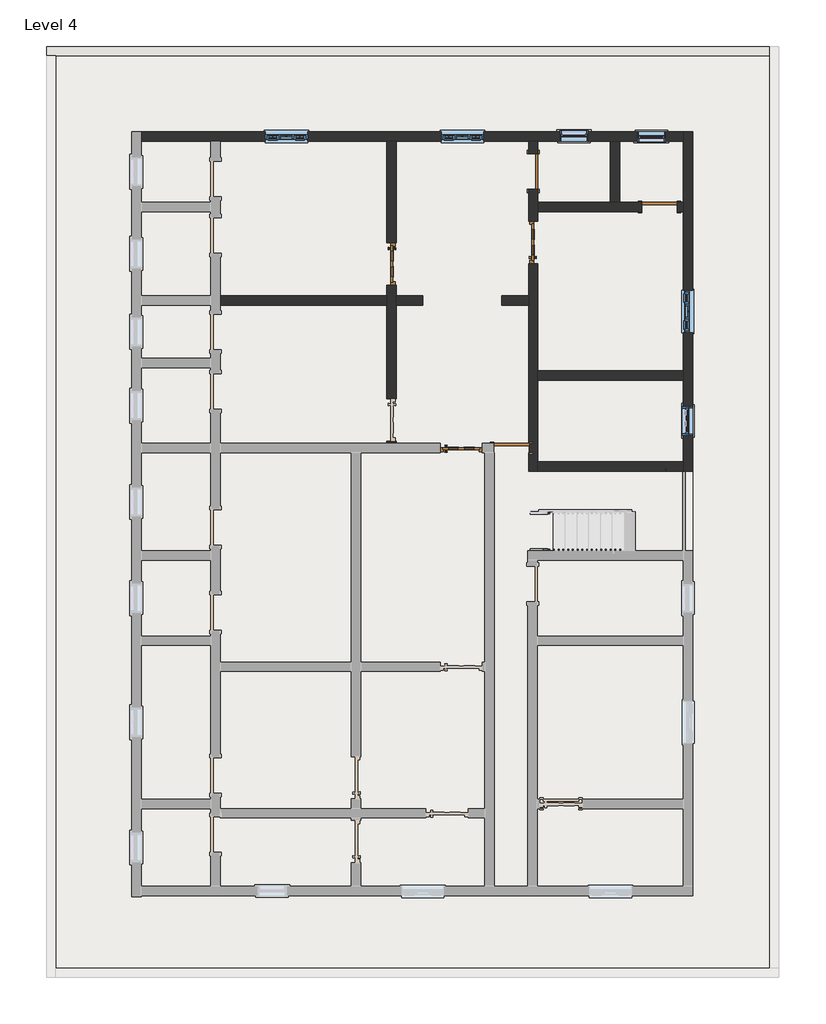
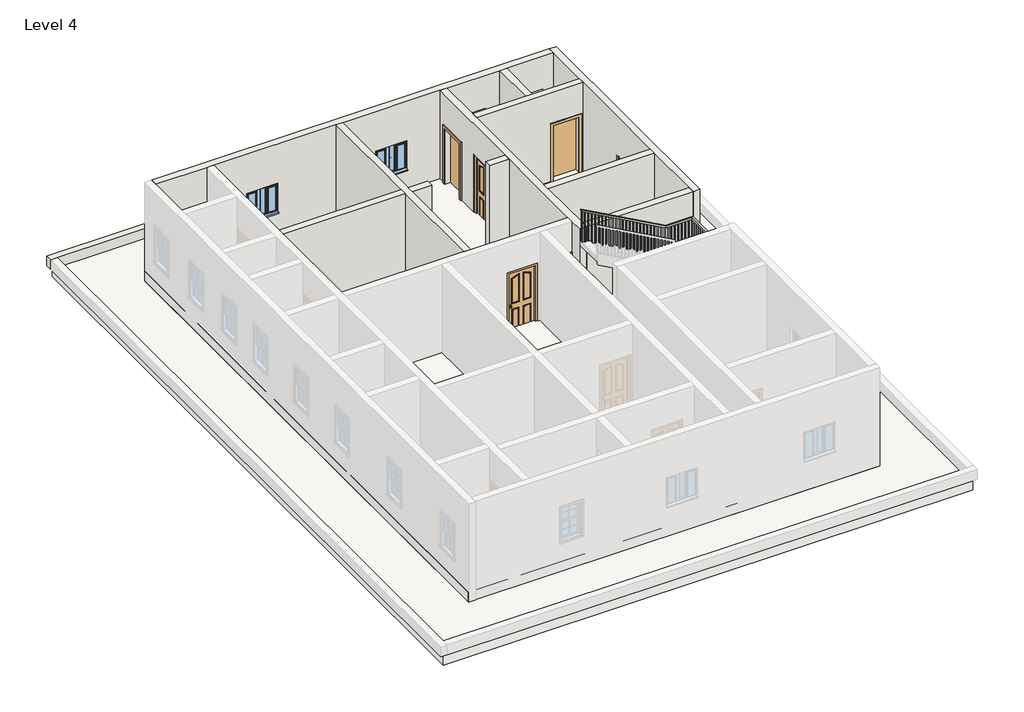
# One storey, part 2 of 3: 11 walls, 6 doors, 6 windows, 2 slabs, 1 railing, 1 roof.
# Revit data of these elements (continued)
# Type "Windows_Tpl_w-Glazing_Cross-Bars : 910x910mm" (continued)
#   Cavity Closer Depth = 0' - 3.34646"
#   Vis - Glazing Bars = yes
#   Vis - Cavity Closers = yes
#   Define Thermal Properties by = 1
#   Material Trim = Window Frame
#   Material Glazing Bars = Window Frame
#   Material Glass = Glass
#   Material Frame = Window Frame
#   Wall Closure = (empty or 0)
# Elements 1, 2, 3 (IfcDoor, "Doors_ExtSgl_12 : 910x2110mm")
#   Phase Created = New Construction
#   Materials on its faces: "Door - Panel", "Door - Handle", "Door - Frame/Mullion", "Door - Glazing"
# Elements 4, 5, 6 (IfcDoor, "Single-Flush : 30\" x 80\"")
#   Phase Created = New Construction
#   Materials on its faces: "Door - Frame", "Door - Panel"
# Element 7 (IfcRailing, "Handrail - Rectangular")
#   Phase Created = New Construction
# Element 8 (IfcRoof, "Generic - 12\"")
#   built-in parameter 1001705 = 31 (stored number, unit not read)
#   built-in parameter 1001710 = 33615
#   Phase Created = New Construction
#   Materials on its faces: "Default Roof"
# Element 9 (IfcSlab, "Generic - 12\"")
#   Height Offset From Level = 0' - 0"
#   Phase Created = New Construction
#   Materials on its faces: "Default Floor"
# Element 10 (IfcSlab, "Generic - 12\"")
#   Height Offset From Level = 0' - 0"
#   Phase Created = New Construction
#   Materials on its faces: "Default Floor", "Tile, Porcelain, 4in"
# Elements 11, 12, 13, 14, 15, 16, 17, 18 (IfcWall, "4.5\"")
#   Top Offset = 0' - 0"
#   Base Offset = 0' - 0"
#   wall height = 10' - 0"
#   Phase Created = New Construction
#   Base Constraint = Level 4
#   Top Constraint = Level 5
#   Materials on its faces: "Default Wall"
# Element 19 (IfcWall, "4.5\"")
#   Top Offset = 0' - 0"
#   Base Offset = 0' - 0"
#   Unconnected Height = 1' - 0"
#   wall height = 1' - 0"
#   Phase Created = New Construction
#   Base Constraint = Level 4
#   Materials on its faces: "Default Wall"
# Elements 20, 21 (IfcWall, "Generic - 9\"")
#   Top Offset = 0' - 0"
#   Base Offset = 0' - 0"
#   wall height = 10' - 0"
#   Phase Created = New Construction
#   Base Constraint = Level 4
#   Top Constraint = Level 5
#   Materials on its faces: "Default Wall", "Tile, Porcelain, 4in"
# Element 22 (IfcWindow, "Window-Double-Hung : 24\" x 42\"")
#   Mark = "71"
#   Window Inset = 0' - 0"
#   Interior Wall Closure = 0' - 1 1/2"
#   Frame Extension = 0' - 1 1/4"
#   Exterior Wall Closure = 0' - 0 1/2"
#   Interior Trim Visibility = yes
#   Indicator Visibility = yes
#   Exterior Trim Visibility = yes
#   Phase Created = New Construction
#   Materials on its faces: "Wood - Stained", "Glass", "Clad - White"
# Element 23 (IfcWindow, "Window-Double-Hung : 24\" x 42\"")
#   Mark = "72"
#   Window Inset = 0' - 0"
#   Interior Wall Closure = 0' - 1 1/2"
#   Frame Extension = 0' - 1 1/4"
#   Exterior Wall Closure = 0' - 0 1/2"
#   Interior Trim Visibility = yes
#   Indicator Visibility = yes
#   Exterior Trim Visibility = yes
#   Phase Created = New Construction
#   Materials on its faces: "Wood - Stained", "Glass", "Clad - White"
# Element 24 (IfcWindow, "Window-Double-Hung : 24\" x 42\"")
#   Mark = "73"
#   Window Inset = 0' - 0"
#   Interior Wall Closure = 0' - 1 1/2"
#   Frame Extension = 0' - 1 1/4"
#   Exterior Wall Closure = 0' - 0 1/2"
#   Interior Trim Visibility = yes
#   Indicator Visibility = yes
#   Exterior Trim Visibility = yes
#   Phase Created = New Construction
#   Materials on its faces: "Wood - Stained", "Glass", "Clad - White"
# Element 25 (IfcWindow, "Windows_Tpl_w-Glazing_Cross-Bars : 910x910mm")
#   Mark = "59"
#   Phase Created = New Construction
#   Materials on its faces: "Window Frame", "Glass"
# Element 26 (IfcWindow, "Windows_Tpl_w-Glazing_Cross-Bars : 910x910mm")
#   Mark = "60"
#   Phase Created = New Construction
#   Materials on its faces: "Window Frame", "Glass"
# Element 27 (IfcWindow, "Windows_Tpl_w-Glazing_Cross-Bars : 910x910mm")
#   Mark = "74"
#   Phase Created = New Construction
#   Materials on its faces: "Window Frame", "Glass"
# Materials
#   "Door - Glazing": colour RGB 0 0 255, transparency 0.75
#   "Door - Panel": class "Wood", colour RGB 210 159 95, transparency 0, Cost = 0
#   "Door - Frame/Mullion": class "Wood", colour RGB 212 179 113, transparency 0
#   "Door - Handle": colour RGB 246 240 166, transparency 0
#   "Door - Frame": colour RGB 118 70 51, transparency 0, Cost = 0
#   "Wood - Stained": class "Wood", colour RGB 224 178 126, transparency 0, Cost = 0
#   "Clad - White": class "Wood", colour RGB 242 242 238, transparency 0, Cost = 0
#   "Glass": class "Glass", colour RGB 0 128 192, transparency 0.75, Description = "Soda Lime Glass", Cost = 0
#   "Window Frame": colour RGB 249 249 249, transparency 0
#   "Default Roof": colour RGB 88 101 114, transparency 0, Cost = 0
#   "Default Floor": colour RGB 128 128 128, transparency 0, Cost = 0
#   "Tile, Porcelain, 4in": class "Generic", colour RGB 89 87 158, transparency 0, Description = "Porcelain tile, 4\", white", Cost = 0
#   "Default Wall": colour RGB 128 128 128, transparency 0, Cost = 0
